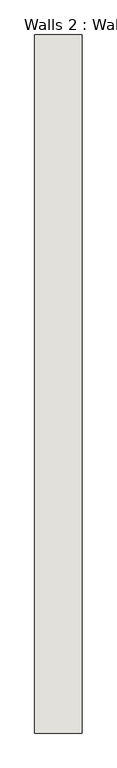
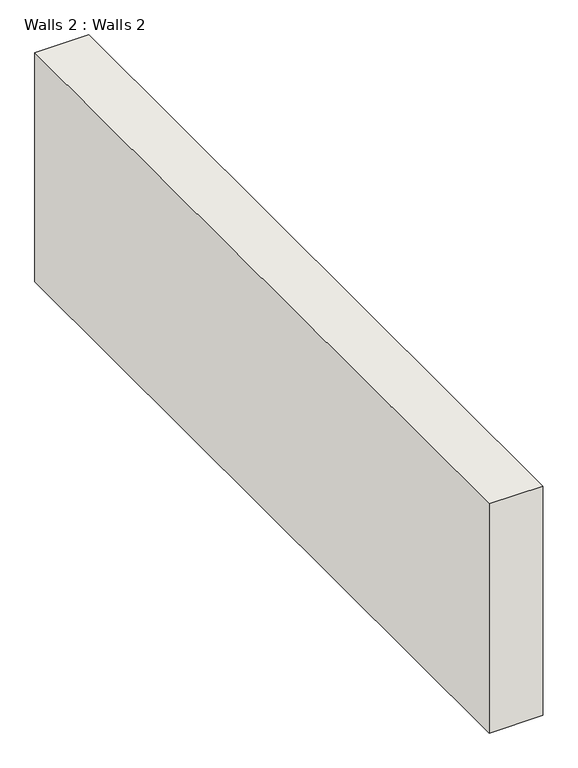
"""IFC4 building model written with IfcOpenShell, lengths in millimetres: wall geometry, Walls 2 : Walls 2."""

from ifc_helpers import new_model, si_unit, frame, origin, place, context, project, spatial, polyline, outline, extrude, source, transform, mapped, element, save


def walls_2_walls_2_0f297521(model_context):
    return source(origin(), model_context, "Body", "SweptSolid", [
        extrude(outline(polyline([(3817.9688099, -1197.7139512), (3817.9688099, -4551.3888327), (3589.3688099, -4551.3888327), (3589.3688099, -1197.7139512), (3817.9688099, -1197.7139512)])), frame((0.0, 0.0, 6587.697392), z_axis=(0.0, 0.0, 1.0), x_axis=(1.0, 0.0, 0.0)), (0.0, 0.0, 1.0), 1032.302608),
    ])


if __name__ == "__main__":
    model = new_model("IFC4")
    model_context = context("Model", 3, world=origin())
    ifc_project = project(units=[si_unit("LENGTHUNIT", "METRE", prefix="MILLI")], contexts=[model_context])
    site = spatial("IfcSite", under=ifc_project)
    building = spatial("IfcBuilding", under=site)
    placement = place(None, origin())
    walls_2_walls_2_shape = walls_2_walls_2_0f297521(model_context)
    element("IfcWall", 1, ObjectType="Walls 2 : Walls 2", at=placement, inside=building, context=model_context, shape_type="MappedRepresentation", body=[
        mapped(walls_2_walls_2_shape, transform((0.0, 0.0, 0.0), x_axis=(1.0, 0.0, 0.0), y_axis=(0.0, 1.0, 0.0), z_axis=(0.0, 0.0, 1.0))),
    ])
    save(model, "model.ifc")

# Revit data of these elements
# Element 1 (IfcWall, "Walls 2 : Walls 2")
#   Materials on its faces: "Default Wall"
# Materials
#   "Default Wall": colour RGB 128 128 128, transparency 0
